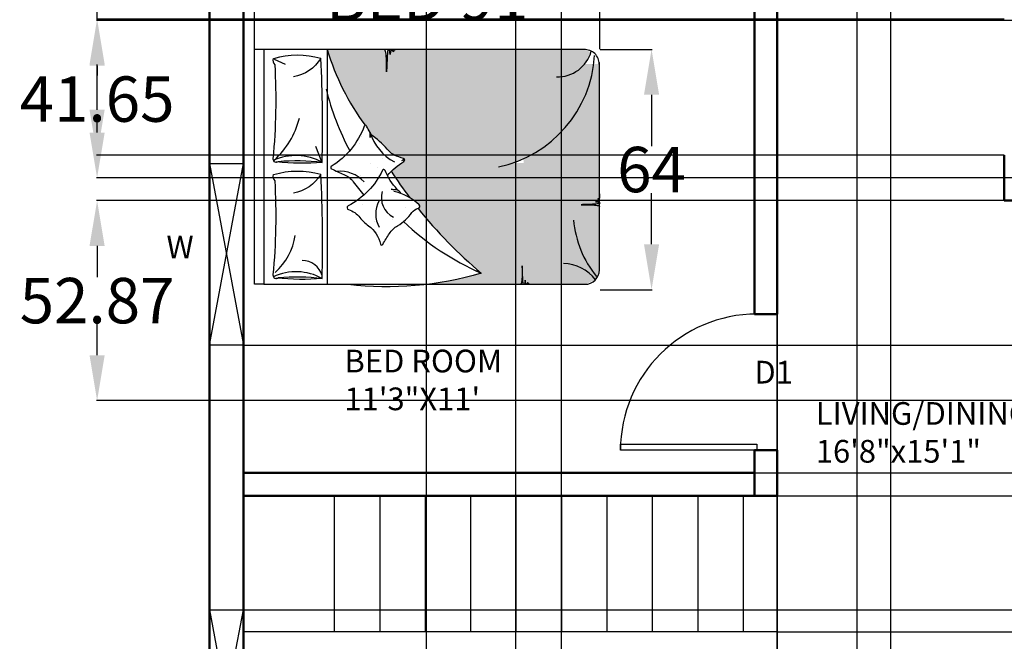
# Model space of a CAD drawing. Units: inches. Extents: x -77 to 516, y -119 to 536.
# Tile 6 of 11: x -36 to 224, y 159 to 323. Entities that reach past the tile are written whole.
import ezdxf

# ---------------------------------------------------------------- set-up
doc = ezdxf.new("R2010")
doc.units = ezdxf.units.IN
doc.header["$MEASUREMENT"] = 0
for name, color, linetype, lineweight in [('A-ANNO-DIMS', 2, 'Continuous', 18), ('A-AREA-IDEN', 170, 'Continuous', 25), ('doors', 6, 'Continuous', 25), ('furniture', 119, 'Continuous', 18), ('steps', 20, 'Continuous', 25), ('text', 170, 'Continuous', 18), ('walls', 40, 'Continuous', 50), ('windows', 1, 'Continuous', 25)]:
    doc.layers.add(name, color=color, linetype=linetype, lineweight=lineweight)
doc.layers.add('FMCHAIR', color=2, linetype='Continuous')
doc.layers.add('HID', color=11, linetype='Continuous')
doc.styles.get("Standard").update_dxf_attribs({"font": 'arial.ttf'})
doc.dimstyles.get("Standard").update_dxf_attribs({"dimtxt": 12, "dimasz": 12, "dimexe": 0.18, "dimexo": 0.0625, "dimgap": 0.09, "dimtad": 0, "dimtih": 1, "dimtoh": 1, "dimdec": 1, "dimzin": 0, "dimdsep": 46, "dimlunit": 4, "dimtxsty": 'Standard', "dimcen": 0.09, "dimadec": 0, "dimazin": 0, "dimtfac": 1, "dimtdec": 1, "dimtofl": 0, "dimtmove": 0, "dimatfit": 3, "dimfxl": 1, "dimtolj": 1, "dimtzin": 0, "dimarcsym": 0})

# ---------------------------------------------------------------- blocks, each defined once
blk = doc.blocks.new('*U2')
for p, q in [((0, 0), (0, -6)), ((40, 0), (40, -6))]:
    blk.add_line(p, q)
blk.add_lwpolyline([(0, 0), (0, 40), (1.75, 40), (1.75, 0)], close=True)
blk.add_arc((0, 0), 40, 0, 90)
blk = doc.blocks.new('*X6')
at = {"color": 0}
for p, q in [((3155.9, 8182.9), (3155.9, 8182.9)), ((3147.8, 8143.4), (3147.8, 8143.4)), ((3283, 8049.6), (3283, 8049.6)), ((3209.5, 8023.9), (3209.5, 8023.9)), ((3251.6, 7997), (3251.6, 7997)), ((3154.1, 7950.7), (3154.1, 7950.7))]:
    blk.add_line(p, q, dxfattribs=at)
blk = doc.blocks.new('*X3')
at = {"color": 0}
for p, q in [((3163, 7776.2), (3163, 7776.2)), ((3422.2, 7761.3), (3422.2, 7761.3)), ((3244.3, 7698.6), (3244.3, 7698.6)), ((3340.3, 7689.4), (3340.3, 7689.4)), ((3236.2, 7675.7), (3236.2, 7675.7))]:
    blk.add_line(p, q, dxfattribs=at)
blk = doc.blocks.new('*X4')
at = {"color": 0}
for p, q in [((3155.9, 8182.9), (3155.9, 8182.9)), ((3139.8, 7939.7), (3139.8, 7939.7))]:
    blk.add_line(p, q, dxfattribs=at)
blk = doc.blocks.new('*X5')
at = {"color": 0}
for p, q in [((3155.9, 8182.9), (3155.9, 8182.9)), ((3139.8, 7939.7), (3139.8, 7939.7))]:
    blk.add_line(p, q, dxfattribs=at)
blk = doc.blocks.new('A$C74474F55')
at = {"layer": 'HID'}
h = blk.add_hatch(dxfattribs=at)
h.set_pattern_fill('SWAMP', color=256, scale=0.05, angle=90, style=0)
h.set_pattern_definition([(270, (-17.63342, -3.553806), (0.04330127, -0.025), [0.00625, -0.04375]), (360, (-17.633422, -3.55693), (0.04330127, 0.025), [0.003125, -0.08347754]), (360, (-17.633422, -3.557712), (0.04330127, 0.025), [0.0025, -0.08410254]), (360, (-17.633422, -3.55615), (0.04330127, 0.025), [0.0025, -0.08410254]), (330, (-17.63342, -3.558494), (0.04330127, 0.025), [0.002, -0.048]), (30, (-17.63342, -3.55537), (2e-11, 0.05), [0.002, -0.048])])
h.paths.add_polyline_path([(1.3153, 0.4546), (1.3153, 1.2689), (1.3045, 1.2693), (1.2905, 1.2698), (1.2792, 1.2703), (1.2715, 1.2706), (1.2685, 1.2708), (1.2711, 1.2709), (1.2784, 1.271), (1.2894, 1.271), (1.3031, 1.271), (1.3153, 1.2712), (1.3153, 1.5955, 0.070745), (0.9502, 1.3987, -0.37626), (0.9456, 1.3906, -0.016811), (0.9066, 1.3696, -0.006874), (0.9057, 1.3691, 0.114631), (0.8849, 1.3514, -0.055725), (0.7962, 1.2557, 0.103757), (0.7727, 1.2248, 0.049789), (0.753, 1.1702, -0.658965), (0.7351, 1.1673, 0.009041), (0.7258, 1.1815), (0.7258, 0.5174, 0.023342), (0.7509, 0.4546)])
h.paths.add_polyline_path([(1.3153, 0.0359), (1.3153, 0.4546), (0.7509, 0.4546, 0.258611)], flags=16)
h.paths.add_polyline_path([(1.3865, 0.0523), (1.4017, 0.0936), (1.4017, 0.4546), (1.3153, 0.4546), (1.3153, 0.0906, 0.096956)])
h.paths.add_polyline_path([(1.4017, 0.4546), (1.4017, 1.2566), (1.3989, 1.2541), (1.3947, 1.2523), (1.3901, 1.2515), (1.3867, 1.2511), (1.3832, 1.2508), (1.3798, 1.2506), (1.3768, 1.2504), (1.3745, 1.2503), (1.3729, 1.2502), (1.3723, 1.25), (1.373, 1.2498), (1.3746, 1.2494), (1.377, 1.249), (1.38, 1.2486), (1.3834, 1.2481), (1.3868, 1.2475), (1.3902, 1.2469), (1.3946, 1.2459), (1.3983, 1.2444), (1.4005, 1.2423), (1.3994, 1.2396), (1.3972, 1.2372), (1.3944, 1.2348), (1.3918, 1.2327), (1.3906, 1.2317), (1.3896, 1.2309), (1.3891, 1.2302), (1.389, 1.2299), (1.3893, 1.2297), (1.39, 1.2297), (1.3909, 1.2297), (1.3937, 1.2299), (1.3967, 1.2294), (1.3984, 1.2269), (1.3993, 1.223), (1.3994, 1.2214), (1.399, 1.224), (1.3986, 1.2259), (1.398, 1.2274), (1.3973, 1.2285), (1.3965, 1.2292), (1.3955, 1.2296), (1.3944, 1.2298), (1.3932, 1.2298), (1.392, 1.2298), (1.3894, 1.2296), (1.3887, 1.23), (1.3908, 1.2319), (1.3933, 1.2339), (1.3948, 1.2351), (1.3963, 1.2364), (1.3976, 1.2377), (1.3988, 1.2389), (1.3996, 1.2401), (1.4, 1.2412), (1.4, 1.2422), (1.3996, 1.2431), (1.3988, 1.244), (1.3974, 1.2448), (1.3956, 1.2455), (1.3931, 1.2462), (1.3902, 1.2469), (1.3868, 1.2475), (1.3834, 1.2481), (1.38, 1.2486), (1.377, 1.249), (1.3732, 1.2497), (1.3721, 1.2501), (1.3745, 1.2503), (1.3768, 1.2504), (1.3798, 1.2506), (1.3832, 1.2508), (1.3867, 1.2511), (1.3901, 1.2515), (1.3932, 1.252), (1.3958, 1.2528), (1.3979, 1.2537), (1.3996, 1.2547), (1.4008, 1.2558), (1.4017, 1.2569), (1.4017, 1.2614), (1.4007, 1.2623), (1.3988, 1.2631), (1.3957, 1.2639), (1.391, 1.2647), (1.3845, 1.2654), (1.3759, 1.2661), (1.3648, 1.2668), (1.3512, 1.2674), (1.3359, 1.2681), (1.32, 1.2687), (1.3153, 1.2689), (1.3153, 0.4546)])
h.paths.add_polyline_path([(1.3634, 1.2728), (1.3749, 1.2739), (1.3839, 1.2754), (1.3909, 1.2772), (1.396, 1.2794), (1.3996, 1.2819), (1.4017, 1.2846), (1.4017, 1.6243), (1.4016, 1.6243, 0.015447), (1.3153, 1.5955), (1.3153, 1.2712), (1.3184, 1.2712), (1.3343, 1.2715), (1.3496, 1.272)])
h.paths.add_polyline_path([(0.7258, 0.4546), (0.7258, 1.1815, 0.042174), (0.6758, 1.2427, 0.017541), (0.5183, 1.1326, -0.05563), (0.4756, 1.0761, -0.589988), (0.4553, 1.0813, 0.007526), (0.4547, 1.0833, 0.049398), (0.0682, 0.7063, -0.041143), (0.0017, 1.0299), (0.0017, 0.4738), (0.0034, 0.4716), (0.0064, 0.4695), (0.0107, 0.4676), (0.0165, 0.4661), (0.024, 0.4649), (0.0335, 0.464), (0.045, 0.4634), (0.0578, 0.4629), (0.071, 0.4627), (0.0838, 0.4625), (0.0952, 0.4625), (0.1044, 0.4625), (0.1105, 0.4624), (0.1126, 0.4623), (0.1102, 0.4621), (0.1038, 0.4619), (0.0943, 0.4615), (0.0827, 0.4611), (0.0698, 0.4606), (0.0565, 0.4601), (0.0437, 0.4595), (0.0324, 0.4589), (0.0232, 0.4584), (0.016, 0.4578), (0.0106, 0.4572), (0.0067, 0.4566), (0.0041, 0.4559), (0.0025, 0.4552), (0.0018, 0.4546)])
h.paths.add_polyline_path([(0.7258, 0.0023), (0.7258, 0.4546), (0.0017, 0.4546), (0.0017, 0.0888), (0.027, 0.0276), (0.0483, 0.0191), (0.0882, 0.0023), (0.4673, 0.0023), (0.4694, 0.0052), (0.4712, 0.0095), (0.4727, 0.0154), (0.4739, 0.0229), (0.4748, 0.0324), (0.4755, 0.0439), (0.4759, 0.0567), (0.4762, 0.0699), (0.4763, 0.0827), (0.4764, 0.0941), (0.4764, 0.1033), (0.4764, 0.1094), (0.4765, 0.1115), (0.4767, 0.1091), (0.477, 0.1027), (0.4773, 0.0932), (0.4778, 0.0816), (0.4783, 0.0687), (0.4788, 0.0554), (0.4793, 0.0426), (0.4799, 0.0313), (0.4805, 0.022), (0.481, 0.0148), (0.4816, 0.0094), (0.4823, 0.0056), (0.4829, 0.003), (0.4832, 0.0023), (0.4899, 0.0023), (0.4899, 0.0023), (0.4908, 0.0037), (0.4915, 0.0055), (0.4922, 0.0077), (0.4926, 0.0102), (0.493, 0.0131), (0.4932, 0.016), (0.4934, 0.0188), (0.4935, 0.0212), (0.4937, 0.0244), (0.4939, 0.0252), (0.4944, 0.0227), (0.495, 0.0186), (0.4955, 0.0158), (0.4959, 0.0129), (0.4965, 0.0102), (0.497, 0.0077), (0.4976, 0.0057), (0.4982, 0.0041), (0.4989, 0.003), (0.4996, 0.0023), (0.502, 0.0023), (0.5021, 0.0023), (0.5031, 0.003), (0.5041, 0.0039), (0.5052, 0.0051), (0.5062, 0.0063), (0.5073, 0.0076), (0.5089, 0.0096), (0.5109, 0.0119), (0.5107, 0.0081), (0.5107, 0.0077), (0.5107, 0.0067), (0.5109, 0.0057), (0.5112, 0.0049), (0.5118, 0.0042), (0.5127, 0.0036), (0.5139, 0.0031), (0.5156, 0.0027), (0.5177, 0.0025), (0.5203, 0.0023), (0.5208, 0.0023)])
h.paths.add_polyline_path([(1.3153, 0.0023), (1.3153, 0.0359, -0.258611), (0.7509, 0.4546), (0.7258, 0.4546), (0.7258, 0.0023)])
at = {"layer": 'FMCHAIR'}
for p, q in [((0.0017, 2.0023), (0.0017, 2.0573)), ((0.0017, 2.0573), (1.4017, 2.0573)), ((1.4017, 2.0023), (1.4017, 2.0573)), ((1.4017, 2.0023), (0.0017, 2.0023)), ((0.0017, 2.0023), (0.0017, 0.0888)), ((1.4017, 0.0936), (1.4017, 2.0023)), ((1.344, 1.9405), (1.3145, 1.8748)), ((1.4016, 1.6243), (0.0017, 1.6243))]:
    blk.add_line(p, q, dxfattribs=at)
for points in [[(0.6558, 1.9468, 0.267769), (0.6186, 1.9372, -0.037739), (0.058, 1.948, 0.684696), (0.0417, 1.9156, -0.060702), (0.0363, 1.6551, -0.046649), (0.0393, 1.9264, -1.318436)], [(0.6558, 1.6631, 0.144019), (0.6541, 1.9447, 0.248643)], [(1.3487, 1.9468, 0.267769), (1.3115, 1.9372, -0.037739), (0.7509, 1.948, 0.684696), (0.7346, 1.9156, -0.060702), (0.7292, 1.6551, -0.046649), (0.7322, 1.9264, -1.318436)], [(0.7418, 1.9405, 0.143972), (0.992, 1.7907, 1.292232)], [(1.3487, 1.6631, 0.144019), (1.347, 1.9447, 0.248643)], [(0.0363, 1.6551, 0.021276), (0.6558, 1.6631, -0.206383), (0.5456, 1.8257, 0.237198)], [(0.7292, 1.6551, 0.021276), (1.3487, 1.6631, -0.206383), (1.2385, 1.8257, 0.237198)], [(0.6517, 1.2658, -0.069098), (0.7351, 1.1673, 0.658965), (0.753, 1.1702, -0.049789), (0.7727, 1.2248, -0.103757), (0.7962, 1.2557, 0.055725), (0.8849, 1.3514, -0.11866), (0.9066, 1.3696, 0.016811), (0.9456, 1.3906, 0.70791), (0.9457, 1.404, -0.16964), (0.7051, 1.6004, 0.664036), (0.6909, 1.5983, 0.023706), (0.6569, 1.5253, -0.134834), (0.6136, 1.4691, 0.012748), (0.5343, 1.406)], [(0.0682, 0.7063, -0.099958), (0, 1.4994)], [(0.5425, 1.1832, 0.263265), (0.5648, 1.216, -0.026108), (0.5685, 1.2431, 0.027613), (0.5675, 1.2072, -0.089259), (0.6816, 1.2795, 0.662242), (0.6823, 1.2947, -0.162037), (0.4689, 1.5004, 0.676499), (0.4471, 1.4982, -0.160513), (0.4002, 1.4294, 0.07473), (0.3513, 1.3788, -0.187721), (0.2417, 1.3067, 0.70791), (0.2402, 1.2934, -0.010003), (0.3044, 1.2536, -0.113819), (0.3514, 1.205, 0.099539), (0.4293, 1.1198, -0.173425), (0.4553, 1.0813, 0.589988), (0.4756, 1.0761, 0.137312), (0.5558, 1.2284, 0.137312)]]:
    blk.add_lwpolyline(points, format="xyb", dxfattribs=at)
for points in [[(0.7322, 1.6576), (0.8244, 1.6933)], [(1.3996, 1.2183), (1.3994, 1.2214), (1.399, 1.224), (1.3986, 1.2259), (1.398, 1.2274), (1.3973, 1.2285), (1.3965, 1.2292), (1.3955, 1.2296), (1.3944, 1.2298), (1.3932, 1.2298), (1.392, 1.2298), (1.3909, 1.2297), (1.39, 1.2297), (1.3893, 1.2297), (1.389, 1.2299), (1.3891, 1.2302), (1.3896, 1.2309), (1.3906, 1.2317), (1.3918, 1.2327), (1.3933, 1.2339), (1.3948, 1.2351), (1.3963, 1.2364), (1.3976, 1.2377), (1.3988, 1.2389), (1.3996, 1.2401), (1.4, 1.2412), (1.4, 1.2422), (1.3996, 1.2431), (1.3988, 1.244), (1.3974, 1.2448), (1.3956, 1.2455), (1.3931, 1.2462), (1.3902, 1.2469), (1.3868, 1.2475), (1.3834, 1.2481), (1.38, 1.2486), (1.377, 1.249), (1.3746, 1.2494), (1.373, 1.2498), (1.3723, 1.25), (1.3729, 1.2502), (1.3745, 1.2503), (1.3768, 1.2504), (1.3798, 1.2506), (1.3832, 1.2508), (1.3867, 1.2511), (1.3901, 1.2515), (1.3932, 1.252), (1.3958, 1.2528), (1.3979, 1.2537), (1.3996, 1.2547), (1.4008, 1.2558), (1.4017, 1.257), (1.4022, 1.2581), (1.4023, 1.2593), (1.4022, 1.2604), (1.4018, 1.2614), (1.4007, 1.2623), (1.3988, 1.2631), (1.3957, 1.2639), (1.391, 1.2647), (1.3845, 1.2654), (1.3759, 1.2661), (1.3648, 1.2668), (1.3512, 1.2674), (1.3359, 1.2681), (1.32, 1.2687), (1.3045, 1.2693), (1.2905, 1.2698), (1.2792, 1.2703), (1.2715, 1.2706), (1.2685, 1.2708), (1.2711, 1.2709), (1.2784, 1.271), (1.2894, 1.271), (1.3031, 1.271), (1.3184, 1.2712), (1.3343, 1.2715), (1.3496, 1.272), (1.3634, 1.2728), (1.3749, 1.2739), (1.3839, 1.2754), (1.3909, 1.2772), (1.396, 1.2794), (1.3996, 1.2819), (1.4007, 1.2833)], [(0.0034, 0.4185), (0.0036, 0.4212), (0.0039, 0.4233), (0.0042, 0.4249), (0.0047, 0.4262), (0.0053, 0.427), (0.006, 0.4276), (0.0068, 0.428), (0.0078, 0.4281), (0.0088, 0.4282), (0.0098, 0.4281), (0.0107, 0.4281), (0.0114, 0.428), (0.012, 0.4281), (0.0123, 0.4282), (0.0122, 0.4285), (0.0117, 0.429), (0.0109, 0.4297), (0.0099, 0.4306), (0.0087, 0.4316), (0.0074, 0.4326), (0.0062, 0.4337), (0.005, 0.4347), (0.0041, 0.4358), (0.0034, 0.4367), (0.0031, 0.4376), (0.003, 0.4385), (0.0034, 0.4392), (0.0041, 0.44), (0.0052, 0.4406), (0.0068, 0.4412), (0.0088, 0.4418), (0.0113, 0.4424), (0.014, 0.4429), (0.0169, 0.4434), (0.0197, 0.4438), (0.0222, 0.4442), (0.0242, 0.4445), (0.0256, 0.4448), (0.0261, 0.445), (0.0257, 0.4451), (0.0244, 0.4452), (0.0224, 0.4453), (0.0199, 0.4455), (0.0171, 0.4456), (0.0142, 0.4459), (0.0114, 0.4462), (0.0088, 0.4467), (0.0066, 0.4473), (0.0048, 0.448), (0.0034, 0.4489), (0.0024, 0.4498), (0.0017, 0.4508), (0.0013, 0.4518), (0.0011, 0.4527), (0.0012, 0.4536), (0.0016, 0.4545), (0.0025, 0.4552), (0.0041, 0.4559), (0.0067, 0.4566), (0.0106, 0.4572), (0.016, 0.4578), (0.0232, 0.4584), (0.0324, 0.4589), (0.0437, 0.4595), (0.0565, 0.4601), (0.0698, 0.4606), (0.0827, 0.4611), (0.0943, 0.4615), (0.1038, 0.4619), (0.1102, 0.4621), (0.1126, 0.4623), (0.1105, 0.4624), (0.1044, 0.4625), (0.0952, 0.4625), (0.0838, 0.4625), (0.071, 0.4627), (0.0578, 0.4629), (0.045, 0.4634), (0.0335, 0.464), (0.024, 0.4649), (0.0165, 0.4661), (0.0107, 0.4676), (0.0064, 0.4695), (0.0034, 0.4716), (0.0025, 0.4727)], [(0.5417, 0.0025), (0.5333, 0.0023), (0.5276, 0.0022), (0.5235, 0.0022), (0.5203, 0.0023), (0.5177, 0.0025), (0.5156, 0.0027), (0.5139, 0.0031), (0.5127, 0.0036), (0.5118, 0.0042), (0.5112, 0.0049), (0.5109, 0.0057), (0.5107, 0.0067), (0.5107, 0.0077), (0.5107, 0.0086), (0.5108, 0.0096), (0.5108, 0.0103), (0.5108, 0.0109), (0.5106, 0.0112), (0.5103, 0.0111), (0.5098, 0.0106), (0.5091, 0.0098), (0.5082, 0.0088), (0.5073, 0.0076), (0.5062, 0.0063), (0.5052, 0.0051), (0.5041, 0.0039), (0.5031, 0.003), (0.5021, 0.0023), (0.5012, 0.0019), (0.5004, 0.0019), (0.4996, 0.0023), (0.4989, 0.003), (0.4982, 0.0041), (0.4976, 0.0057), (0.497, 0.0077), (0.4965, 0.0102), (0.4959, 0.0129), (0.4955, 0.0158), (0.495, 0.0186), (0.4947, 0.0211), (0.4943, 0.0231), (0.4941, 0.0245), (0.4939, 0.025), (0.4937, 0.0246), (0.4936, 0.0232), (0.4935, 0.0212), (0.4934, 0.0188), (0.4932, 0.016), (0.493, 0.0131), (0.4926, 0.0102), (0.4922, 0.0077), (0.4915, 0.0055), (0.4908, 0.0037), (0.4899, 0.0023), (0.489, 0.0013), (0.4881, 0.0005), (0.4871, 0.0001), (0.4861, 0), (0.4852, 0.0001), (0.4844, 0.0005), (0.4836, 0.0014), (0.4829, 0.003), (0.4823, 0.0056), (0.4816, 0.0094), (0.481, 0.0148), (0.4805, 0.022), (0.4799, 0.0313), (0.4793, 0.0426), (0.4788, 0.0554), (0.4783, 0.0687), (0.4778, 0.0816), (0.4773, 0.0932), (0.477, 0.1027), (0.4767, 0.1091), (0.4765, 0.1115), (0.4764, 0.1094), (0.4764, 0.1033), (0.4764, 0.0941), (0.4763, 0.0827), (0.4762, 0.0699), (0.4759, 0.0567), (0.4755, 0.0439), (0.4748, 0.0324), (0.4739, 0.0229), (0.4727, 0.0154), (0.4712, 0.0095), (0.4694, 0.0052), (0.4672, 0.0023), (0.4661, 0.0014)], [(0.0882, 0.0023), (1.3249, 0.0023)]]:
    blk.add_lwpolyline(points, dxfattribs=at)
for centre, radius, start, end in [((-0.2415, 1.8109), 0.3185, 330.71255, 25.00895), ((0.4514, 1.8109), 0.3185, 330.71255, 25.00895), ((0.3528, 2.1867), 0.3765, 222.01178, 260.96348), ((0.0166, 1.7766), 0.1282, 287.40732, 358.51286), ((1.5564, 0.0535), 1.625, 103.90497, 117.81692), ((1.8245, 0.2133), 1.473, 106.68314, 126.40962), ((0.4777, 1.5498), 0.1986, 313.20348, 5.05559), ((1.0005, 1.0782), 0.3061, 107.86019, 151.51221), ((0.8877, 1.4681), 0.1003, 263.675, 280.88198), ((0.8903, 1.4005), 0.0349, 246.83517, 297.72181), ((0.4227, 1.1722), 0.1634, 62.61037, 119.36102), ((0.5198, 1.1712), 0.1311, 74.0372, 153.45361), ((2.165, -1.0566), 2.7394, 122.93136, 126.95099), ((0.7222, 1.1686), 0.0208, 343.79673, 40.45661), ((1.5564, 0.0535), 1.625, 136.58872, 156.3156), ((0.733, 1.1738), 0.0143, 309.7097, 355.9506), ((2.165, -1.0566), 2.7394, 128.63292, 139.94485), ((1.4108, 0.7544), 0.7248, 191.95357, 266.49279), ((1.4488, 0.2531), 0.2103, 178.64103, 254.46876), ((-0.1244, 0.2231), 0.2505, 307.85533, 358.44053), ((0.4383, -0.4561), 0.6148, 94.95248, 129.36976), ((0.0882, 0.0888), 0.0865, 180, 270), ((1.3153, 0.0896), 0.0865, 270, 3.53765)]:
    blk.add_arc(centre, radius, start, end, dxfattribs=at)
at = {"layer": 'FMCHAIR', "xscale": 0.001, "yscale": 0.001, "zscale": 0.001, "rotation": 270}
for name in ['*X3', '*X4', '*X5', '*X6']:
    blk.add_blockref(name, (-7.2998, 4.5776), dxfattribs=at)
blk = doc.blocks.new('WIN-48IN')
for p, q in [((0, 0), (9, 48)), ((0, 48), (9, 0))]:
    blk.add_line(p, q)
blk.add_lwpolyline([(0, 48), (9, 48), (9, 0), (0, 0)], close=True)
blk = doc.blocks.new('*D28')
at = {"layer": 'A-ANNO-DIMS', "color": 0, "lineweight": -2, "transparency": 16777216}
for p, q in [((25.71, 315.63), (25.71, 329.43)), ((37.71, 329.25), (44.48, 329.25)), ((104.89, 329.25), (98.13, 329.25)), ((116.89, 315.63), (116.89, 329.43))]:
    blk.add_line(p, q, dxfattribs=at)
at = {"layer": 'A-ANNO-DIMS', "color": 0, "transparency": 16777216}
for points in [[(37.71, 331.25), (37.71, 327.25), (25.71, 329.25)], [(104.89, 331.25), (104.89, 327.25), (116.89, 329.25)]]:
    blk.add_solid(points, dxfattribs=at)
at = {"layer": 'Defpoints', "color": 0, "transparency": 16777216}
for p in [(25.71, 329.25), (25.71, 315.57), (116.89, 315.57)]:
    blk.add_point(p, dxfattribs=at)
at = {"layer": 'A-ANNO-DIMS', "color": 0, "transparency": 16777216, "insert": (71.3, 329.25), "char_height": 12, "attachment_point": 5}
blk.add_mtext('\\A1;BED 91', dxfattribs=at)
blk = doc.blocks.new('*D29')
at = {"layer": 'A-ANNO-DIMS', "color": 0, "lineweight": -2, "transparency": 16777216}
for p, q in [((116.95, 315.57), (130.75, 315.57)), ((130.57, 303.57), (130.57, 290.02)), ((130.57, 264.04), (130.57, 277.59)), ((116.95, 252.04), (130.75, 252.04))]:
    blk.add_line(p, q, dxfattribs=at)
at = {"layer": 'A-ANNO-DIMS', "color": 0, "transparency": 16777216}
for points in [[(128.57, 303.57), (132.57, 303.57), (130.57, 315.57)], [(128.57, 264.04), (132.57, 264.04), (130.57, 252.04)]]:
    blk.add_solid(points, dxfattribs=at)
at = {"layer": 'Defpoints', "color": 0, "transparency": 16777216}
for p in [(116.89, 315.57), (130.57, 315.57), (116.89, 252.04)]:
    blk.add_point(p, dxfattribs=at)
at = {"layer": 'A-ANNO-DIMS', "color": 0, "transparency": 16777216, "insert": (130.57, 283.8), "char_height": 12, "attachment_point": 5}
blk.add_mtext('\\A1;64', dxfattribs=at)
blk = doc.blocks.new('*D39')
at = {"layer": 'A-ANNO-DIMS', "color": 0, "lineweight": -2, "transparency": 16777216}
for p, q in [((22.75, 485.53), (22.75, -111.24)), ((71.05, 485.53), (71.05, -111.24)), ((34.75, -111.06), (59.05, -111.06)), ((71.05, -111.06), (83.05, -111.06))]:
    blk.add_line(p, q, dxfattribs=at)
at = {"layer": 'A-ANNO-DIMS', "color": 0, "transparency": 16777216}
for points in [[(34.75, -109.06), (34.75, -113.06), (22.75, -111.06)], [(59.05, -109.06), (59.05, -113.06), (71.05, -111.06)]]:
    blk.add_solid(points, dxfattribs=at)
at = {"layer": 'Defpoints', "color": 0, "transparency": 16777216}
for p in [(22.75, 485.59), (71.05, 485.59), (71.05, -111.06)]:
    blk.add_point(p, dxfattribs=at)
at = {"layer": 'A-ANNO-DIMS', "color": 0, "transparency": 16777216, "insert": (108.33, -111.06), "char_height": 12, "attachment_point": 5}
blk.add_mtext('\\A1;48.295', dxfattribs=at)
blk = doc.blocks.new('*D40')
at = {"layer": 'A-ANNO-DIMS', "color": 0, "lineweight": -2, "transparency": 16777216}
for p, q in [((163.750061, 485.5259), (163.750061, -111.2416)), ((184.750061, 485.5259), (184.750061, -111.2416)), ((151.750061, -111.0616), (139.750061, -111.0616)), ((196.750061, -111.0616), (208.750061, -111.0616))]:
    blk.add_line(p, q, dxfattribs=at)
at = {"layer": 'A-ANNO-DIMS', "color": 0, "transparency": 16777216}
for points in [[(151.750061, -109.0616), (151.750061, -113.0616), (163.750061, -111.0616)], [(196.750061, -109.0616), (196.750061, -113.0616), (184.750061, -111.0616)]]:
    blk.add_solid(points, dxfattribs=at)
at = {"layer": 'Defpoints', "color": 0, "transparency": 16777216}
for p in [(163.750061, 485.5884), (184.750061, 485.5884), (184.750061, -111.0616)]:
    blk.add_point(p, dxfattribs=at)
at = {"layer": 'A-ANNO-DIMS', "color": 0, "transparency": 16777216, "insert": (174.250061, -111.0616), "char_height": 12, "attachment_point": 5}
blk.add_mtext('\\A1;21', dxfattribs=at)
blk = doc.blocks.new('*D42')
at = {"layer": 'A-ANNO-DIMS', "color": 0, "lineweight": -2, "transparency": 16777216}
for p, q in [((454.4, 197.59), (454.4, 209.59)), ((454.4, 209.59), (466.4, 209.59)), ((22.81, 197.59), (454.58, 197.59)), ((454.4, 179.41), (454.4, 185.59)), ((22.81, 167.41), (454.58, 167.41))]:
    blk.add_line(p, q, dxfattribs=at)
at = {"layer": 'A-ANNO-DIMS', "color": 0, "transparency": 16777216}
for points in [[(452.4, 185.59), (456.4, 185.59), (454.4, 197.59)], [(452.4, 179.41), (456.4, 179.41), (454.4, 167.41)]]:
    blk.add_solid(points, dxfattribs=at)
at = {"layer": 'Defpoints', "color": 0, "transparency": 16777216}
for p in [(22.75, 197.59), (454.4, 197.59), (22.75, 167.41)]:
    blk.add_point(p, dxfattribs=at)
at = {"layer": 'A-ANNO-DIMS', "color": 0, "transparency": 16777216, "insert": (486.75, 209.59), "char_height": 12, "attachment_point": 5}
blk.add_mtext('\\A1;30.18', dxfattribs=at)
blk = doc.blocks.new('*D43')
at = {"layer": 'A-ANNO-DIMS', "color": 0, "lineweight": -2, "transparency": 16777216}
for p, q in [((454.4, 237.36), (454.4, 249.36)), ((454.4, 249.36), (466.4, 249.36)), ((22.81, 237.36), (454.58, 237.36)), ((454.4, 215.59), (454.4, 225.36)), ((22.81, 203.59), (454.58, 203.59))]:
    blk.add_line(p, q, dxfattribs=at)
at = {"layer": 'A-ANNO-DIMS', "color": 0, "transparency": 16777216}
for points in [[(452.4, 225.36), (456.4, 225.36), (454.4, 237.36)], [(452.4, 215.59), (456.4, 215.59), (454.4, 203.59)]]:
    blk.add_solid(points, dxfattribs=at)
at = {"layer": 'Defpoints', "color": 0, "transparency": 16777216}
for p in [(22.75, 237.36), (454.4, 237.36), (22.75, 203.59)]:
    blk.add_point(p, dxfattribs=at)
at = {"layer": 'A-ANNO-DIMS', "color": 0, "transparency": 16777216, "insert": (491.44, 249.36), "char_height": 12, "attachment_point": 5}
blk.add_mtext('\\A1;33.775', dxfattribs=at)
blk = doc.blocks.new('*D46')
at = {"layer": 'A-ANNO-DIMS', "color": 0, "lineweight": -2, "transparency": 16777216}
for p, q in [((-15.9, 323.59), (-15.9, 335.59)), ((-15.9, 335.59), (-3.9, 335.59)), ((223.69, 323.59), (-16.08, 323.59)), ((-15.9, 299.59), (-15.9, 311.59)), ((223.69, 287.59), (-16.08, 287.59))]:
    blk.add_line(p, q, dxfattribs=at)
at = {"layer": 'A-ANNO-DIMS', "color": 0, "transparency": 16777216}
for points in [[(-17.9, 311.59), (-13.9, 311.59), (-15.9, 323.59)], [(-17.9, 299.59), (-13.9, 299.59), (-15.9, 287.59)]]:
    blk.add_solid(points, dxfattribs=at)
at = {"layer": 'Defpoints', "color": 0, "transparency": 16777216}
for p in [(-15.9, 323.59), (223.75, 323.59), (223.75, 287.59)]:
    blk.add_point(p, dxfattribs=at)
at = {"layer": 'A-ANNO-DIMS', "color": 0, "transparency": 16777216, "insert": (4.78, 335.59), "char_height": 12, "attachment_point": 5}
blk.add_mtext('\\A1;36', dxfattribs=at)
blk = doc.blocks.new('*D47')
at = {"layer": 'A-ANNO-DIMS', "color": 0, "lineweight": -2, "transparency": 16777216}
for p, q in [((364.69, 275.59), (-16.08, 275.59)), ((-15.9, 263.59), (-15.9, 255.37)), ((-15.9, 234.71), (-15.9, 242.93)), ((364.69, 222.71), (-16.08, 222.71))]:
    blk.add_line(p, q, dxfattribs=at)
at = {"layer": 'A-ANNO-DIMS', "color": 0, "transparency": 16777216}
for points in [[(-17.9, 263.59), (-13.9, 263.59), (-15.9, 275.59)], [(-17.9, 234.71), (-13.9, 234.71), (-15.9, 222.71)]]:
    blk.add_solid(points, dxfattribs=at)
at = {"layer": 'Defpoints', "color": 0, "transparency": 16777216}
for p in [(-15.9, 275.59), (364.75, 275.59), (364.75, 222.71)]:
    blk.add_point(p, dxfattribs=at)
at = {"layer": 'A-ANNO-DIMS', "color": 0, "transparency": 16777216, "insert": (-15.9, 249.15), "char_height": 12, "attachment_point": 5}
blk.add_mtext('\\A1;52.87', dxfattribs=at)
blk = doc.blocks.new('*D48')
at = {"layer": 'A-ANNO-DIMS', "color": 0, "lineweight": -2, "transparency": 16777216}
for p, q in [((364.69, 323.24), (-16.08, 323.24)), ((-15.9, 311.24), (-15.9, 308.63)), ((-15.9, 293.59), (-15.9, 296.2)), ((364.69, 281.59), (-16.08, 281.59))]:
    blk.add_line(p, q, dxfattribs=at)
at = {"layer": 'A-ANNO-DIMS', "color": 0, "transparency": 16777216}
for points in [[(-17.9, 311.24), (-13.9, 311.24), (-15.9, 323.24)], [(-17.9, 293.59), (-13.9, 293.59), (-15.9, 281.59)]]:
    blk.add_solid(points, dxfattribs=at)
at = {"layer": 'Defpoints', "color": 0, "transparency": 16777216}
for p in [(-15.9, 323.24), (364.75, 323.24), (364.75, 281.59)]:
    blk.add_point(p, dxfattribs=at)
at = {"layer": 'A-ANNO-DIMS', "color": 0, "transparency": 16777216, "insert": (-15.9, 302.42), "char_height": 12, "attachment_point": 5}
blk.add_mtext('\\A1;41.65', dxfattribs=at)
blk = doc.blocks.new('*D53')
at = {"layer": 'A-ANNO-DIMS', "color": 0, "lineweight": -2, "transparency": 16777216}
for p, q in [((163.75, 95.65), (163.75, 525.13)), ((175.75, 524.95), (181.75, 524.95)), ((193.75, 95.65), (193.75, 525.13)), ((193.75, 524.95), (205.75, 524.95))]:
    blk.add_line(p, q, dxfattribs=at)
at = {"layer": 'A-ANNO-DIMS', "color": 0, "transparency": 16777216}
for points in [[(175.75, 526.95), (175.75, 522.95), (163.75, 524.95)], [(181.75, 526.95), (181.75, 522.95), (193.75, 524.95)]]:
    blk.add_solid(points, dxfattribs=at)
at = {"layer": 'Defpoints', "color": 0, "transparency": 16777216}
for p in [(193.75, 524.95), (163.75, 95.59), (193.75, 95.59)]:
    blk.add_point(p, dxfattribs=at)
at = {"layer": 'A-ANNO-DIMS', "color": 0, "transparency": 16777216, "insert": (214.41, 524.95), "char_height": 12, "attachment_point": 5}
blk.add_mtext('\\A1;30', dxfattribs=at)
blk = doc.blocks.new('*D54')
at = {"layer": 'A-ANNO-DIMS', "color": 0, "lineweight": -2, "transparency": 16777216}
for p, q in [((82.75, 524.95), (70.75, 524.95)), ((94.75, 120.65), (94.75, 525.13)), ((106.75, 120.65), (106.75, 525.13)), ((118.75, 524.95), (130.75, 524.95))]:
    blk.add_line(p, q, dxfattribs=at)
at = {"layer": 'A-ANNO-DIMS', "color": 0, "transparency": 16777216}
for points in [[(82.75, 526.95), (82.75, 522.95), (94.75, 524.95)], [(118.75, 526.95), (118.75, 522.95), (106.75, 524.95)]]:
    blk.add_solid(points, dxfattribs=at)
at = {"layer": 'Defpoints', "color": 0, "transparency": 16777216}
for p in [(106.75, 524.95), (94.75, 120.59), (106.75, 120.59)]:
    blk.add_point(p, dxfattribs=at)
at = {"layer": 'A-ANNO-DIMS', "color": 0, "transparency": 16777216, "insert": (138.81, 524.95), "char_height": 12, "attachment_point": 5}
blk.add_mtext('\\A1;12', dxfattribs=at)
blk = doc.blocks.new('*D55')
at = {"layer": 'A-ANNO-DIMS', "color": 0, "lineweight": -2, "transparency": 16777216}
for p, q in [((454.4, 197.59), (454.4, 209.59)), ((454.4, 209.59), (466.4, 209.59)), ((163.81, 197.59), (454.58, 197.59)), ((454.4, 173.59), (454.4, 185.59)), ((163.81, 161.59), (454.58, 161.59))]:
    blk.add_line(p, q, dxfattribs=at)
at = {"layer": 'A-ANNO-DIMS', "color": 0, "transparency": 16777216}
for points in [[(452.4, 185.59), (456.4, 185.59), (454.4, 197.59)], [(452.4, 173.59), (456.4, 173.59), (454.4, 161.59)]]:
    blk.add_solid(points, dxfattribs=at)
at = {"layer": 'Defpoints', "color": 0, "transparency": 16777216}
for p in [(163.75, 197.59), (454.4, 197.59), (163.75, 161.59)]:
    blk.add_point(p, dxfattribs=at)
at = {"layer": 'A-ANNO-DIMS', "color": 0, "transparency": 16777216, "insert": (475.08, 209.59), "char_height": 12, "attachment_point": 5}
blk.add_mtext('\\A1;36', dxfattribs=at)
blk = doc.blocks.new('*D56')
at = {"layer": 'A-ANNO-DIMS', "color": 0, "lineweight": -2, "transparency": 16777216}
for p, q in [((454.4, 215.59), (454.4, 227.59)), ((454.4, 227.59), (466.4, 227.59)), ((157.81, 203.59), (454.58, 203.59)), ((157.81, 197.59), (454.58, 197.59)), ((454.4, 185.59), (454.4, 173.59))]:
    blk.add_line(p, q, dxfattribs=at)
at = {"layer": 'A-ANNO-DIMS', "color": 0, "transparency": 16777216}
for points in [[(452.4, 215.59), (456.4, 215.59), (454.4, 203.59)], [(452.4, 185.59), (456.4, 185.59), (454.4, 197.59)]]:
    blk.add_solid(points, dxfattribs=at)
at = {"layer": 'Defpoints', "color": 0, "transparency": 16777216}
for p in [(157.75, 203.59), (454.4, 203.59), (157.75, 197.59)]:
    blk.add_point(p, dxfattribs=at)
at = {"layer": 'A-ANNO-DIMS', "color": 0, "transparency": 16777216, "insert": (470.45, 227.59), "char_height": 12, "attachment_point": 5}
blk.add_mtext('\\A1;6', dxfattribs=at)

msp = doc.modelspace()

# ---------------------------------------------------------------- linework, layer by layer
at = {"layer": 'steps'}
for p, q in [((46.7501, 197.5884), (46.7501, 161.5884)), ((58.7501, 197.5884), (58.7501, 161.5884)), ((70.7501, 197.5884), (70.7501, 161.5884)), ((82.7501, 197.5884), (82.7501, 161.5884)), ((94.7501, 197.5884), (94.7501, 161.5884)), ((106.7501, 197.5884), (106.7501, 161.5884)), ((118.7501, 197.5884), (118.7501, 161.5884)), ((130.7501, 197.5884), (130.7501, 161.5884)), ((142.7501, 197.5884), (142.7501, 161.5884)), ((154.7501, 197.5884), (154.7501, 161.5884)), ((163.7501, 161.5884), (163.7501, 197.5884)), ((163.7501, 161.5884), (22.7501, 161.5884))]:
    msp.add_line(p, q, dxfattribs=at)
at = {"layer": 'walls'}
for p, q in [((163.7501, 341.5884), (163.7501, 245.5884)), ((22.7501, 335.5884), (22.7501, 23.5884)), ((157.7501, 335.5884), (157.7501, 245.5884)), ((223.7501, 287.5884), (223.7501, 275.5884)), ((364.7501, 275.5884), (223.7501, 275.5884)), ((163.7501, 245.5884), (157.7501, 245.5884)), ((163.7501, 209.5884), (157.7501, 209.5884)), ((157.7501, 209.5884), (157.7501, 197.5884)), ((163.7501, 209.5884), (163.7501, 197.5884)), ((157.7501, 203.5884), (22.7501, 203.5884)), ((163.7501, 197.5884), (22.7501, 197.5884))]:
    msp.add_line(p, q, dxfattribs=at)
msp.add_lwpolyline([(373.7501, 131.5884), (373.7501, 494.5884), (13.7501, 494.5884), (13.7501, 14.5884), (239.7501, 14.5884)], dxfattribs=at)

# ---------------------------------------------------------------- block references
at = {"layer": 'doors', "xscale": 0.9000000000000026, "yscale": 0.9000000000000026, "zscale": 0.9000000000000026, "rotation": 90.00000000000055}
msp.add_blockref('*U2', (158.3501, 209.5884), dxfattribs=at)
at = {"layer": 'furniture', "xscale": 44.31992428171801, "yscale": 44.31992428171801, "zscale": 44.31992428171801, "rotation": 90}
msp.add_blockref('A$C74474F55', (116.8925, 253.3817), dxfattribs=at)
at = {"layer": 'windows'}
for p in [(13.75, 237.3636), (13.75, 119.4084)]:
    msp.add_blockref('WIN-48IN', p, dxfattribs=at)

# ---------------------------------------------------------------- texts
at = {"layer": 'A-AREA-IDEN', "char_height": 6, "attachment_point": 1}
for s, insert in [('BED ROOM\\P11\'3"X11\'', (49.4364, 236.179)), ('LIVING/DINING\\P16\'8"x15\'1"', (173.9529, 222.3229))]:
    msp.add_mtext_dynamic_manual_height_columns(s, width=105.041962, gutter_width=1, heights=[0], dxfattribs=dict(at, insert=insert))
at = {"layer": 'text', "char_height": 6, "attachment_point": 1}
for s, insert in [('W', (2.4242, 266.3121)), ('D1', (157.729, 233.2346))]:
    msp.add_mtext_dynamic_manual_height_columns(s, width=105.041962, gutter_width=1, heights=[0], dxfattribs=dict(at, insert=insert))

# ---------------------------------------------------------------- dimensions: what is measured, and where the dimension line sits
at = {"layer": 'A-ANNO-DIMS'}
for base, p1, p2, override, picture, middle in [((106.7501, 524.9457), (94.7501, 120.5884), (106.7501, 120.5884), {"dimdec": 0, "dimlfac": 1, "dimrnd": 0, "dimzin": 0, "dimdsep": 46, "dimlunit": 2}, '*D54', (138.8087, 524.9457)), ((193.7501, 524.9457), (163.7501, 95.5884), (193.7501, 95.5884), {"dimdec": 0, "dimlfac": 1, "dimrnd": 0, "dimzin": 0, "dimdsep": 46, "dimlunit": 2}, '*D53', (214.4103, 524.9457)), ((71.0451, -111.0616), (22.7501, 485.5884), (71.0451, 485.5884), {"dimdec": 3, "dimlfac": 1, "dimrnd": 0, "dimzin": 0, "dimdsep": 46, "dimlunit": 2}, '*D39', (108.3302, -111.0616)), ((184.7501, -111.0616), (163.7501, 485.5884), (184.7501, 485.5884), {"dimdec": 0, "dimlfac": 1, "dimrnd": 0, "dimzin": 0, "dimdsep": 46, "dimlunit": 2}, '*D40', (174.2501, -111.0616))]:
    dim = msp.add_linear_dim(base=base, p1=p1, p2=p2, dimstyle='Standard', override=override, dxfattribs=at)
    dim.commit()
    dim.dimension.update_dxf_attribs({"geometry": picture, "text_midpoint": middle})
dim = msp.add_linear_dim(base=(25.7144, 329.2459), p1=(116.8925, 315.5692), p2=(25.7144, 315.5692), angle=180, text='BED <>', dimstyle='Standard', override={"dimdec": 0, "dimlfac": 1, "dimrnd": 0, "dimzin": 0, "dimdsep": 46, "dimlunit": 2}, dxfattribs=at)
dim.commit()
dim.dimension.update_dxf_attribs({"geometry": '*D28', "text_midpoint": (71.3034, 329.2459)})
for base, p1, p2, override, picture, middle in [((-15.8999, 323.5884), (223.7501, 287.5884), (223.7501, 323.5884), {"dimdec": 0, "dimlfac": 1, "dimrnd": 0, "dimzin": 0, "dimdsep": 46, "dimlunit": 2}, '*D46', (4.7767, 335.5884)), ((-15.8999, 323.2426), (364.7501, 281.5884), (364.7501, 323.2426), {"dimdec": 2, "dimlfac": 1, "dimrnd": 0, "dimzin": 0, "dimdsep": 46, "dimlunit": 2}, '*D48', (-15.8999, 302.4155)), ((130.5692, 315.5692), (116.8925, 252.0371), (116.8925, 315.5692), {"dimdec": 0, "dimlfac": 1, "dimrnd": 0, "dimzin": 0, "dimdsep": 46, "dimlunit": 2}, '*D29', (130.5692, 283.8032)), ((-15.8999, 275.5884), (364.7501, 222.7137), (364.7501, 275.5884), {"dimdec": 2, "dimlfac": 1, "dimrnd": 0, "dimzin": 0, "dimdsep": 46, "dimlunit": 2}, '*D47', (-15.8999, 249.151)), ((454.4001, 237.3631), (22.7501, 203.5884), (22.7501, 237.3631), {"dimdec": 3, "dimlfac": 1, "dimrnd": 0, "dimzin": 0, "dimdsep": 46, "dimlunit": 2}, '*D43', (491.4396, 249.3631)), ((454.4001, 203.5884), (157.7501, 197.5884), (157.7501, 203.5884), {"dimdec": 0, "dimlfac": 1, "dimrnd": 0, "dimzin": 0, "dimdsep": 46, "dimlunit": 2}, '*D56', (470.4519, 227.5884)), ((454.4001, 197.5884), (22.7501, 167.4079), (22.7501, 197.5884), {"dimdec": 2, "dimlfac": 1, "dimrnd": 0, "dimzin": 0, "dimdsep": 46, "dimlunit": 2}, '*D42', (486.7452, 209.5884)), ((454.4001, 197.5884), (163.7501, 161.5884), (163.7501, 197.5884), {"dimdec": 0, "dimlfac": 1, "dimrnd": 0, "dimzin": 0, "dimdsep": 46, "dimlunit": 2}, '*D55', (475.0767, 209.5884))]:
    dim = msp.add_linear_dim(base=base, p1=p1, p2=p2, angle=90, dimstyle='Standard', override=override, dxfattribs=at)
    dim.commit()
    dim.dimension.update_dxf_attribs({"geometry": picture, "text_midpoint": middle})

doc.saveas('drawing.dxf')
